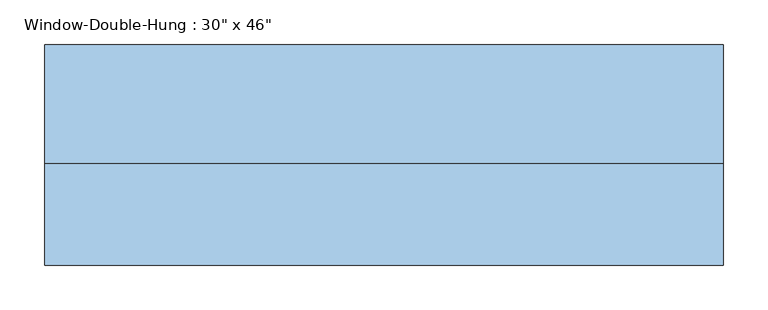
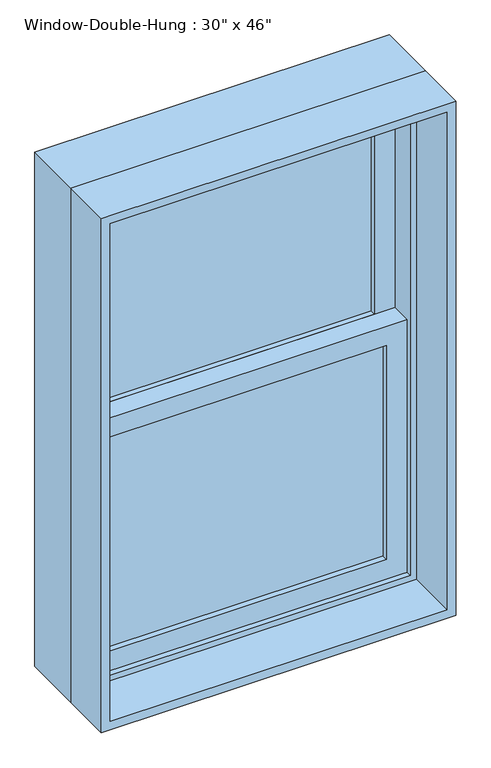
"""IFC4 building model written with IfcOpenShell, lengths in millimetres: window geometry."""

from ifc_helpers import new_model, si_unit, frame, origin, place, context, project, spatial, polyline, outline, extrude, source, transform, mapped, element, save


def window_d400040f(model_context):
    return source(origin(), model_context, "Body", "SweptSolid", [
        extrude(outline(polyline([(304.8, 44.45), (304.8, 38.1), (-304.8, 38.1), (-304.8, 44.45), (304.8, 44.45)])), frame((0.0, 0.0, 990.6), z_axis=(0.0, 0.0, 1.0), x_axis=(1.0, 0.0, 0.0)), (0.0, 0.0, 1.0), 485.775),
        extrude(outline(polyline([(-304.8, 31.75), (304.8, 31.75), (304.8, 25.4), (-304.8, 25.4), (-304.8, 31.75)])), frame((0.0, 0.0, 990.6), z_axis=(0.0, 0.0, 1.0), x_axis=(1.0, 0.0, 0.0)), (0.0, 0.0, 1.0), 485.775),
        extrude(outline(polyline([(304.8, 88.9), (304.8, 82.55), (-304.8, 82.55), (-304.8, 88.9), (304.8, 88.9)])), frame((0.0, 0.0, 1520.825), z_axis=(0.0, 0.0, 1.0), x_axis=(1.0, 0.0, 0.0)), (0.0, 0.0, 1.0), 485.775),
        extrude(outline(polyline([(-304.8, 76.2), (304.8, 76.2), (304.8, 69.85), (-304.8, 69.85), (-304.8, 76.2)])), frame((0.0, 0.0, 1520.825), z_axis=(0.0, 0.0, 1.0), x_axis=(1.0, 0.0, 0.0)), (0.0, 0.0, 1.0), 485.775),
        extrude(outline(polyline([(1520.825, -349.25), (946.15, -349.25), (946.15, 349.25), (1520.825, 349.25), (1520.825, -349.25)]), holes=[polyline([(1476.375, 304.8), (990.6, 304.8), (990.6, -304.8), (1476.375, -304.8), (1476.375, 304.8)])]), frame((0.0, 12.7, 0.0), z_axis=(0.0, 1.0, 0.0), x_axis=(0.0, 0.0, 1.0)), (0.0, 0.0, 1.0), 44.45),
        extrude(outline(polyline([(2051.05, -349.25), (1476.375, -349.25), (1476.375, 349.25), (2051.05, 349.25), (2051.05, -349.25)]), holes=[polyline([(2006.6, 304.8), (1520.825, 304.8), (1520.825, -304.8), (2006.6, -304.8), (2006.6, 304.8)])]), frame((0.0, 57.15, 0.0), z_axis=(0.0, 1.0, 0.0), x_axis=(0.0, 0.0, 1.0)), (0.0, 0.0, 1.0), 44.45),
        extrude(outline(polyline([(2082.8, -381.0), (914.4, -381.0), (914.4, 381.0), (2082.8, 381.0), (2082.8, -381.0)]), holes=[polyline([(2051.05, 349.25), (946.15, 349.25), (946.15, -349.25), (2051.05, -349.25), (2051.05, 349.25)])]), frame((0.0, 0.0, 0.0), z_axis=(0.0, 1.0, 0.0), x_axis=(0.0, 0.0, 1.0)), (0.0, 0.0, 1.0), 133.35),
        extrude(outline(polyline([(2082.8, 381.0), (2082.8, -381.0), (914.4, -381.0), (914.4, 381.0), (2082.8, 381.0)]), holes=[polyline([(2063.75, 361.95), (933.45, 361.95), (933.45, -361.95), (2063.75, -361.95), (2063.75, 361.95)])]), frame((0.0, -114.3, 0.0), z_axis=(0.0, 1.0, 0.0), x_axis=(0.0, 0.0, 1.0)), (0.0, 0.0, 1.0), 114.3),
    ])


if __name__ == "__main__":
    model = new_model("IFC4")
    model_context = context("Model", 3, world=origin())
    ifc_project = project(units=[si_unit("LENGTHUNIT", "METRE", prefix="MILLI")], contexts=[model_context])
    site = spatial("IfcSite", under=ifc_project)
    building = spatial("IfcBuilding", under=site)
    placement = place(None, origin())
    window_shape = window_d400040f(model_context)
    element("IfcWindow", 1, ObjectType="Window-Double-Hung : 30\" x 46\"", at=placement, inside=building, context=model_context, shape_type="MappedRepresentation", body=[
        mapped(window_shape, transform((0.0, 0.0, 0.0), x_axis=(1.0, 0.0, 0.0), y_axis=(0.0, 1.0, 0.0), z_axis=(0.0, 0.0, 1.0))),
    ])
    save(model, "model.ifc")

# Revit data of these elements
# Type "Window-Double-Hung : 30\" x 46\""
#   Type Mark = "13"
#   Fire Rating = "0.5h"
#   Construction Type Id = "DG-DR"
#   Assembly Code = "B2020100"
#   Analytic Construction = "Double glazing - domestic"
#   Wall Thickness [instance default] = 0' - 6"
#   Window Inset [instance default] = 0' - 0"
#   Visual Light Transmittance = 0.81
#   Thermal Resistance (R) = 1.8146 (h·ft²·°F)/BTU
#   Solar Heat Gain Coefficient = 0.76
#   Muntin Width = 2' - 0"
#   Muntin Height = 1' - 7 1/8"
#   Interior Wall Closure [instance default] = 0' - 1 1/2"
#   Rough Width = 2' - 6 1/2"
#   Rough Height = 3' - 10 1/2"
#   Frame Extension [instance default] = 0' - 1 1/4"
#   Exterior Wall Closure [instance default] = 0' - 0 1/2"
#   Extension Jamb [instance default] = 0' - 1 1/2"
#   Heat Transfer Coefficient (U) = 0.5511 BTU/(h·ft²·°F)
#   Height = 3' - 10"
#   Width = 2' - 6"
#   Define Thermal Properties by = 1
#   Top Muntin Visibility = yes
#   Indicator Visibility [instance default] = yes
#   Extension Jamb Visibility [instance default] = yes
#   Interior Trim Visibility [instance default] = yes
#   Exterior Trim Visibility [instance default] = yes
#   Define Thermal Properties by = 1
#   Bottom Muntin Visibility = yes
#   Muntin Pattern = Muntin Pattern_2x2 : Muntin Pattern_2x2
#   Interior Trim Material = Wood - Stained
#   Interior Trim = Trim-Window-Interior-Flat : Picture Frame
#   Exterior Trim Material = Clad - White
#   Exterior Trim = Trim-Window-Exterior-Flat : with Sill
#   Glass Panel Material = Glass
#   Exterior Frame Material = Clad - White
#   Interior Frame Material = Wood - Stained
#   Wall Closure = (empty or 0)
# Element 1 (IfcWindow, "Window-Double-Hung : 30\" x 46\"")
#   Wall Thickness = 0' - 9"
#   Extension Jamb = 0' - 4 1/2"
#   Materials on its faces: "Wood - Stained", "Glass", "Clad - White"
# Materials
#   "Wood - Stained": class "Wood", colour RGB 224 178 126, transparency 0, Cost = 0
#   "Clad - White": class "Wood", colour RGB 242 242 238, transparency 0, Cost = 0
#   "Glass": class "Glass", colour RGB 0 128 192, transparency 0.75, Description = "Soda Lime Glass", Cost = 0
